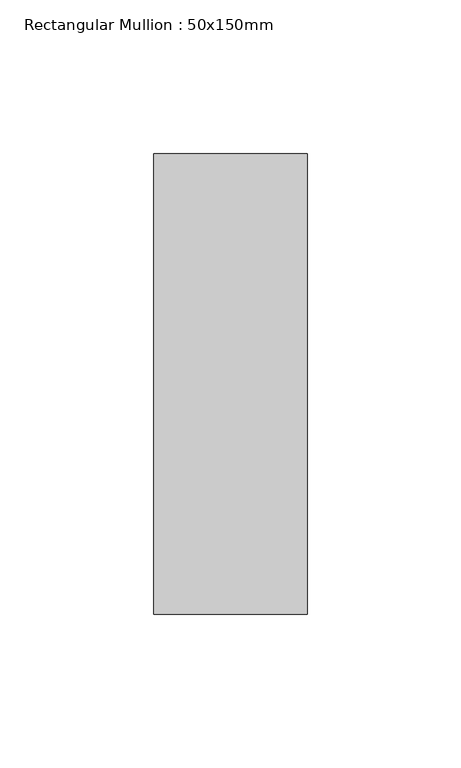
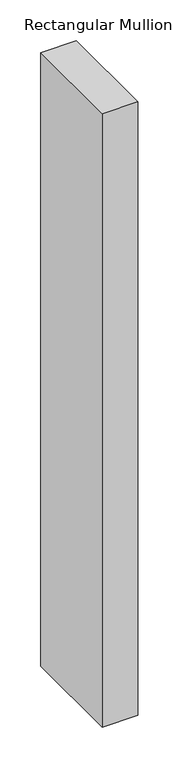
"""IFC4 building model written with IfcOpenShell, lengths in millimetres: member geometry, Rectangular Mullion : 50x150mm."""

from ifc_helpers import new_model, si_unit, frame, origin, place, context, project, spatial, polyline, outline, extrude, source, transform, mapped, element, save


def rectangular_mullion_50x150mm_cc836158(model_context):
    return source(origin(), model_context, "Body", "SweptSolid", [
        extrude(outline(polyline([(0.0, 75.0), (0.0, -75.0), (-50.0, -75.0), (-50.0, 75.0), (0.0, 75.0)])), frame((0.0, 0.0, -914.4), z_axis=(0.0, 0.0, 1.0), x_axis=(1.0, 0.0, 0.0)), (0.0, 0.0, 1.0), 914.4),
    ])


if __name__ == "__main__":
    model = new_model("IFC4")
    model_context = context("Model", 3, world=origin())
    ifc_project = project(units=[si_unit("LENGTHUNIT", "METRE", prefix="MILLI")], contexts=[model_context])
    site = spatial("IfcSite", under=ifc_project)
    building = spatial("IfcBuilding", under=site)
    placement = place(None, origin())
    rectangular_mullion_50x150mm_shape = rectangular_mullion_50x150mm_cc836158(model_context)
    element("IfcMember", 1, ObjectType="Rectangular Mullion : 50x150mm", at=placement, inside=building, context=model_context, shape_type="MappedRepresentation", body=[
        mapped(rectangular_mullion_50x150mm_shape, transform((0.0, 0.0, 0.0), x_axis=(1.0, 0.0, 0.0), y_axis=(0.0, 1.0, 0.0), z_axis=(0.0, 0.0, 1.0))),
    ])
    save(model, "model.ifc")

# Revit data of these elements
# Type "Rectangular Mullion : 50x150mm"
#   Keynote = "H11"
#   built-in parameter 1007304 = 0.492126 (stored number, unit not read)
#   built-in parameter 1007301 = 0.082021 (stored number, unit not read)
#   built-in parameter 1007300 = 0.082021 (stored number, unit not read)
# Element 1 (IfcMember, "Rectangular Mullion : 50x150mm")
#   Materials on its faces: "Aluminium"
# Materials
#   "Aluminium": class "Metal", colour RGB 247 247 247, transparency 0, Description = "Aluminium 6061", Cost = 0
